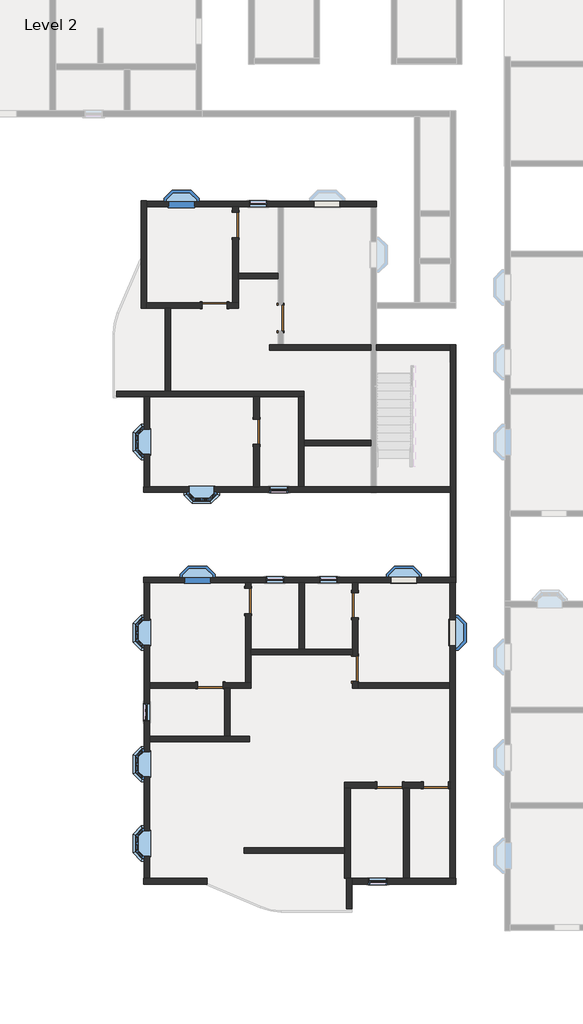
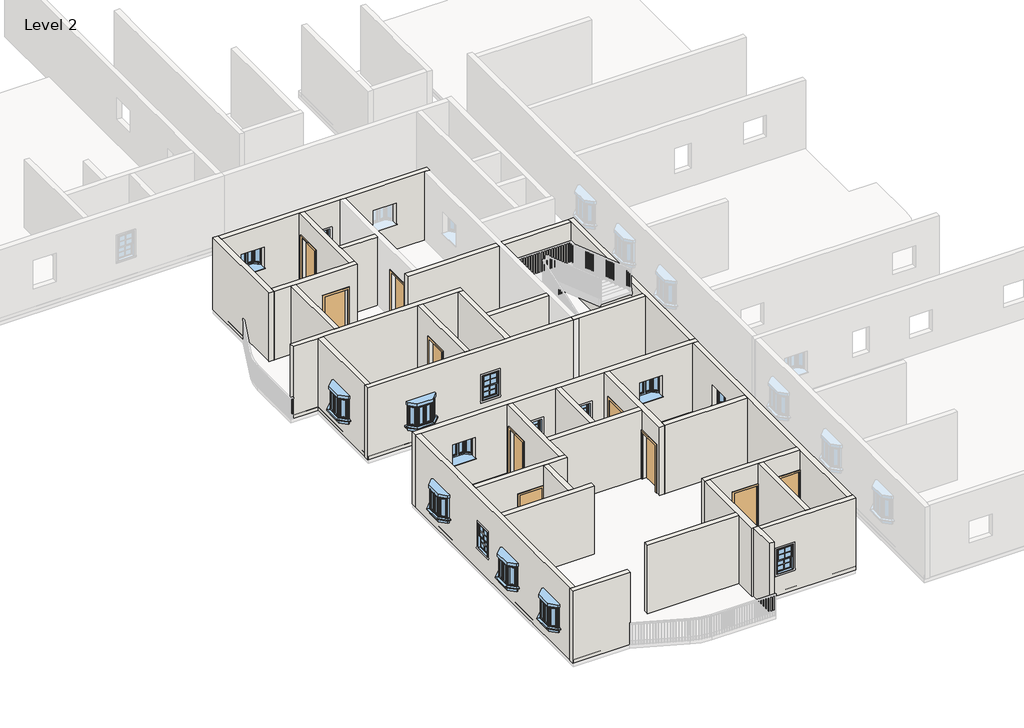
# One storey, part 1 of 14: 32 walls, 15 windows, 10 doors.
"""IFC4 building model written with IfcOpenShell, lengths in millimetres."""

from ifc_helpers import new_model, si_unit, frame, origin, place, context, project, spatial, polyline, outline, extrude, faceted_brep, transform, mapped, element, save
from components import door_54dd4da4, door_719f80de, window_910x910mm_67ef725a, window_8debb0fa

model = new_model("IFC4")

# Units and contexts
model_context = context("Model", 3, world=origin())
ifc_project = project(units=[si_unit("LENGTHUNIT", "METRE", prefix="MILLI")], contexts=[model_context])

# Site, building, storey
site = spatial("IfcSite", under=ifc_project)
building = spatial("IfcBuilding", under=site)
storey = spatial("IfcBuildingStorey", under=building, Name="Level 2", Elevation=3048.0)

# Doors
placement = place(None, origin())
door_shape = door_54dd4da4(model_context)
element("IfcDoor", 1, ObjectType="Single-Flush : 36\" x 84\"", at=placement, inside=storey, context=model_context, shape_type="MappedRepresentation", body=[
    mapped(door_shape, transform((-4626.037215, -17283.4916506, 3048.0), x_axis=(0.0, -1.0, 0.0), y_axis=(1.0, 0.0, 0.0), z_axis=(0.0, 0.0, 1.0))),
])
element("IfcDoor", 2, ObjectType="Single-Flush : 36\" x 84\"", at=placement, inside=storey, context=model_context, shape_type="MappedRepresentation", body=[
    mapped(door_shape, transform((-4626.037215, -14978.4416506, 3048.0), x_axis=(0.0, 1.0, 0.0), y_axis=(-1.0, 0.0, 0.0), z_axis=(0.0, 0.0, 1.0))),
])
element("IfcDoor", 3, ObjectType="Single-Flush : 36\" x 84\"", at=placement, inside=storey, context=model_context, shape_type="MappedRepresentation", body=[
    mapped(door_shape, transform((-9731.437215, -4100.8916506, 3048.0), x_axis=(1.0, 0.0, 0.0), y_axis=(0.0, 1.0, 0.0), z_axis=(0.0, 0.0, 1.0))),
])
element("IfcDoor", 4, ObjectType="Single-Flush : 36\" x 84\"", at=placement, inside=storey, context=model_context, shape_type="MappedRepresentation", body=[
    mapped(door_shape, transform((-7331.137215, -4558.0916506, 3048.0), x_axis=(0.0, -1.0, 0.0), y_axis=(1.0, 0.0, 0.0), z_axis=(0.0, 0.0, 1.0))),
])
door_2_shape = door_719f80de(model_context)
element("IfcDoor", 5, ObjectType="Single-Flush : 36\" x 84\"", at=placement, inside=storey, context=model_context, shape_type="MappedRepresentation", body=[
    mapped(door_2_shape, transform((-9883.837215, -17891.2072331, 3048.0), x_axis=(1.0, 0.0, 0.0), y_axis=(0.0, 1.0, 0.0), z_axis=(0.0, 0.0, 1.0))),
])
element("IfcDoor", 6, ObjectType="Single-Flush : 36\" x 84\"", at=placement, inside=storey, context=model_context, shape_type="MappedRepresentation", body=[
    mapped(door_2_shape, transform((-8512.237215, -14826.0416506, 3048.0), x_axis=(0.0, 1.0, 0.0), y_axis=(-1.0, 0.0, 0.0), z_axis=(0.0, 0.0, 1.0))),
])
element("IfcDoor", 7, ObjectType="Single-Flush : 36\" x 84\"", at=placement, inside=storey, context=model_context, shape_type="MappedRepresentation", body=[
    mapped(door_2_shape, transform((-8207.437215, -8691.9416506, 3048.0), x_axis=(0.0, 1.0, 0.0), y_axis=(-1.0, 0.0, 0.0), z_axis=(0.0, 0.0, 1.0))),
])
element("IfcDoor", 8, ObjectType="Single-Flush : 36\" x 84\"", at=placement, inside=storey, context=model_context, shape_type="MappedRepresentation", body=[
    mapped(door_2_shape, transform((-8969.437215, -1186.2416506, 3048.0), x_axis=(0.0, 1.0, 0.0), y_axis=(-1.0, 0.0, 0.0), z_axis=(0.0, 0.0, 1.0))),
])
element("IfcDoor", 9, ObjectType="Single-Flush : 36\" x 84\"", at=placement, inside=storey, context=model_context, shape_type="MappedRepresentation", body=[
    mapped(door_2_shape, transform((-3374.4891351, -21512.5916506, 3048.0), x_axis=(1.0, 0.0, 0.0), y_axis=(0.0, 1.0, 0.0), z_axis=(0.0, 0.0, 1.0))),
])
element("IfcDoor", 10, ObjectType="Single-Flush : 36\" x 84\"", at=placement, inside=storey, context=model_context, shape_type="MappedRepresentation", body=[
    mapped(door_2_shape, transform((-1698.0891351, -21512.5916506, 3048.0), x_axis=(1.0, 0.0, 0.0), y_axis=(0.0, 1.0, 0.0), z_axis=(0.0, 0.0, 1.0))),
])

# Walls
element("IfcWall", 11, ObjectType="4.5\" p", at=placement, inside=storey, context=model_context, shape_type="Brep", body=[
    faceted_brep([(-9426.637215, -17992.8072331, 5181.6), (-9426.637215, -17992.8072331, 3048.0), (-9375.837215, -17992.8072331, 3048.0), (-9172.637215, -17992.8072331, 3048.0), (-8410.637215, -17992.8072331, 3048.0), (-8410.637215, -17992.8072331, 6096.0), (-9172.637215, -17992.8072331, 6096.0), (-9375.837215, -17992.8072331, 6096.0), (-12087.287215, -17992.8072331, 6096.0), (-12087.287215, -17992.8072331, 3048.0), (-10341.037215, -17992.8072331, 3048.0), (-10341.037215, -17992.8072331, 5181.6), (-8410.637215, -17789.6072331, 3048.0), (-8613.837215, -17789.6072331, 3048.0), (-9426.637215, -17789.6072331, 3048.0), (-9426.637215, -17789.6072331, 5181.6), (-10341.037215, -17789.6072331, 5181.6), (-10341.037215, -17789.6072331, 3048.0), (-12087.287215, -17789.6072331, 3048.0), (-12087.287215, -17789.6072331, 6096.0), (-8613.837215, -17789.6072331, 6096.0), (-8410.637215, -17789.6072331, 6096.0)], [[[0, 1, 2, 3, 4, 5, 6, 7, 8, 9, 10, 11]], [[12, 13, 14, 15, 16, 17, 18, 19, 20, 21]], [[10, 9, 18, 17]], [[4, 3, 2, 1, 14, 13, 12]], [[8, 7, 6, 5, 21, 20, 19]], [[9, 8, 19, 18]], [[5, 4, 12, 21]], [[15, 14, 1, 0]], [[16, 15, 0, 11]], [[17, 16, 11, 10]]]),
])
element("IfcWall", 12, ObjectType="4.5\" p", at=placement, inside=storey, context=model_context, shape_type="Brep", body=[
    faceted_brep([(-8410.637215, -14368.8416506, 5181.6), (-8410.637215, -14368.8416506, 3048.0), (-8410.637215, -14165.6416506, 3048.0), (-8410.637215, -14165.6416506, 6096.0), (-8410.637215, -16572.2916506, 6096.0), (-8410.637215, -16775.4916506, 6096.0), (-8410.637215, -17789.6072331, 6096.0), (-8410.637215, -17789.6072331, 3048.0), (-8410.637215, -16775.4916506, 3048.0), (-8410.637215, -16572.2916506, 3048.0), (-8410.637215, -15283.2416506, 3048.0), (-8410.637215, -15283.2416506, 5181.6), (-8613.837215, -14165.6416506, 3048.0), (-8613.837215, -14368.8416506, 3048.0), (-8613.837215, -14368.8416506, 5181.6), (-8613.837215, -15283.2416506, 5181.6), (-8613.837215, -15283.2416506, 3048.0), (-8613.837215, -17789.6072331, 3048.0), (-8613.837215, -17789.6072331, 6096.0), (-8613.837215, -14165.6416506, 6096.0)], [[[0, 1, 2, 3, 4, 5, 6, 7, 8, 9, 10, 11]], [[12, 13, 14, 15, 16, 17, 18, 19]], [[2, 1, 13, 12]], [[10, 9, 8, 7, 17, 16]], [[6, 5, 4, 3, 19, 18]], [[7, 6, 18, 17]], [[3, 2, 12, 19]], [[14, 13, 1, 0]], [[15, 14, 0, 11]], [[16, 15, 11, 10]]]),
])
element("IfcWall", 13, ObjectType="4.5\" p", at=placement, inside=storey, context=model_context, shape_type="Brep", body=[
    faceted_brep([(-8410.637215, -16775.4916506, 3048.0), (-4727.637215, -16775.4916506, 3048.0), (-4727.637215, -16775.4916506, 6096.0), (-8410.637215, -16775.4916506, 6096.0), (-8410.637215, -16572.2916506, 3048.0), (-8410.637215, -16572.2916506, 6096.0), (-6670.737215, -16572.2916506, 6096.0), (-6467.537215, -16572.2916506, 6096.0), (-4727.637215, -16572.2916506, 6096.0), (-4727.637215, -16572.2916506, 3048.0), (-6467.537215, -16572.2916506, 3048.0), (-6670.737215, -16572.2916506, 3048.0)], [[[0, 1, 2, 3]], [[4, 5, 6, 7, 8, 9, 10, 11]], [[1, 0, 4, 11, 10, 9]], [[3, 2, 8, 7, 6, 5]], [[0, 3, 5, 4]], [[2, 1, 9, 8]]]),
])
element("IfcWall", 14, ObjectType="4.5\" p", at=placement, inside=storey, context=model_context, shape_type="SweptSolid", body=[
    extrude(outline(polyline([(-6670.737215, -16572.2916506), (-6670.737215, -14165.6416506), (-6467.537215, -14165.6416506), (-6467.537215, -16572.2916506), (-6670.737215, -16572.2916506)])), frame((0.0, 0.0, 3048.0), z_axis=(0.0, 0.0, 1.0), x_axis=(1.0, 0.0, 0.0)), (0.0, 0.0, 1.0), 3048.0),
])
element("IfcWall", 15, ObjectType="4.5\" p", at=placement, inside=storey, context=model_context, shape_type="Brep", body=[
    faceted_brep([(-4727.637215, -14165.6416506, 3048.0), (-4727.637215, -14521.2416506, 3048.0), (-4727.637215, -14521.2416506, 5181.6), (-4727.637215, -15435.6416506, 5181.6), (-4727.637215, -15435.6416506, 3048.0), (-4727.637215, -16572.2916506, 3048.0), (-4727.637215, -16775.4916506, 3048.0), (-4727.637215, -16826.2916506, 3048.0), (-4727.637215, -16826.2916506, 5181.6), (-4727.637215, -17740.6916506, 5181.6), (-4727.637215, -17740.6916506, 3048.0), (-4727.637215, -17994.6916506, 3048.0), (-4727.637215, -17994.6916506, 6096.0), (-4727.637215, -16775.4916506, 6096.0), (-4727.637215, -16572.2916506, 6096.0), (-4727.637215, -14165.6416506, 6096.0), (-4524.437215, -14521.2416506, 5181.6), (-4524.437215, -14521.2416506, 3048.0), (-4524.437215, -14165.6416506, 3048.0), (-4524.437215, -14165.6416506, 6096.0), (-4524.437215, -17791.4916506, 6096.0), (-4524.437215, -17994.6916506, 6096.0), (-4524.437215, -17994.6916506, 3048.0), (-4524.437215, -17791.4916506, 3048.0), (-4524.437215, -17740.6916506, 3048.0), (-4524.437215, -17740.6916506, 5181.6), (-4524.437215, -16826.2916506, 5181.6), (-4524.437215, -16826.2916506, 3048.0), (-4524.437215, -15435.6416506, 3048.0), (-4524.437215, -15435.6416506, 5181.6)], [[[0, 1, 2, 3, 4, 5, 6, 7, 8, 9, 10, 11, 12, 13, 14, 15]], [[16, 17, 18, 19, 20, 21, 22, 23, 24, 25, 26, 27, 28, 29]], [[11, 10, 24, 23, 22]], [[28, 27, 7, 6, 5, 4]], [[18, 17, 1, 0]], [[15, 14, 13, 12, 21, 20, 19]], [[0, 15, 19, 18]], [[12, 11, 22, 21]], [[25, 24, 10, 9]], [[26, 25, 9, 8]], [[27, 26, 8, 7]], [[2, 1, 17, 16]], [[3, 2, 16, 29]], [[4, 3, 29, 28]]]),
])
element("IfcWall", 16, ObjectType="4.5\" p", at=placement, inside=storey, context=model_context, shape_type="SweptSolid", body=[
    extrude(outline(polyline([(-4524.437215, -17791.4916506), (-1190.0891351, -17791.4916506), (-1190.0891351, -17994.6916506), (-4524.437215, -17994.6916506), (-4524.437215, -17791.4916506)])), frame((0.0, 0.0, 3048.0), z_axis=(0.0, 0.0, 1.0), x_axis=(1.0, 0.0, 0.0)), (0.0, 0.0, 1.0), 3048.0),
])
element("IfcWall", 17, ObjectType="4.5\" p", at=placement, inside=storey, context=model_context, shape_type="SweptSolid", body=[
    extrude(outline(polyline([(-9375.837215, -19734.5916506), (-9375.837215, -17992.8072331), (-9172.637215, -17992.8072331), (-9172.637215, -19734.5916506), (-9375.837215, -19734.5916506)])), frame((0.0, 0.0, 3048.0), z_axis=(0.0, 0.0, 1.0), x_axis=(1.0, 0.0, 0.0)), (0.0, 0.0, 1.0), 3048.0),
])
element("IfcWall", 18, ObjectType="4.5\" p", at=placement, inside=storey, context=model_context, shape_type="Brep", body=[
    faceted_brep([(-12087.287215, -19937.7916506, 3048.0), (-8455.087215, -19937.7916506, 3048.0), (-8455.087215, -19937.7916506, 6096.0), (-12087.287215, -19937.7916506, 6096.0), (-12087.287215, -19734.5916506, 3048.0), (-12087.287215, -19734.5916506, 6096.0), (-9375.837215, -19734.5916506, 6096.0), (-9172.637215, -19734.5916506, 6096.0), (-8455.087215, -19734.5916506, 6096.0), (-8455.087215, -19734.5916506, 3048.0), (-9172.637215, -19734.5916506, 3048.0), (-9375.837215, -19734.5916506, 3048.0)], [[[0, 1, 2, 3]], [[4, 5, 6, 7, 8, 9, 10, 11]], [[1, 0, 4, 11, 10, 9]], [[2, 1, 9, 8]], [[3, 2, 8, 7, 6, 5]], [[0, 3, 5, 4]]]),
])
element("IfcWall", 19, ObjectType="4.5\" p", at=placement, inside=storey, context=model_context, shape_type="Brep", body=[
    faceted_brep([(-13293.787215, -7421.9416506, 3048.0), (-12290.487215, -7421.9416506, 3048.0), (-12087.287215, -7421.9416506, 3048.0), (-8309.037215, -7421.9416506, 3048.0), (-8105.837215, -7421.9416506, 3048.0), (-6689.787215, -7421.9416506, 3048.0), (-6486.587215, -7421.9416506, 3048.0), (-6486.587215, -7421.9416506, 6096.0), (-6689.787215, -7421.9416506, 6096.0), (-8105.837215, -7421.9416506, 6096.0), (-8309.037215, -7421.9416506, 6096.0), (-12087.287215, -7421.9416506, 6096.0), (-12290.487215, -7421.9416506, 6096.0), (-13293.787215, -7421.9416506, 6096.0), (-13293.787215, -7218.7416506, 3048.0), (-13293.787215, -7218.7416506, 6096.0), (-11528.487215, -7218.7416506, 6096.0), (-11325.287215, -7218.7416506, 6096.0), (-6486.587215, -7218.7416506, 6096.0), (-6486.587215, -7218.7416506, 3048.0), (-11325.287215, -7218.7416506, 3048.0), (-11528.487215, -7218.7416506, 3048.0)], [[[0, 1, 2, 3, 4, 5, 6, 7, 8, 9, 10, 11, 12, 13]], [[14, 15, 16, 17, 18, 19, 20, 21]], [[6, 5, 4, 3, 2, 1, 0, 14, 21, 20, 19]], [[13, 12, 11, 10, 9, 8, 7, 18, 17, 16, 15]], [[0, 13, 15, 14]], [[7, 6, 19, 18]]]),
])
element("IfcWall", 20, ObjectType="4.5\" p", at=placement, inside=storey, context=model_context, shape_type="Brep", body=[
    faceted_brep([(-12201.587215, -4202.4916506, 3048.0), (-12201.587215, -3999.2916506, 3048.0), (-12201.587215, -525.8416506, 3048.0), (-12201.587215, -322.6416506, 3048.0), (-12201.587215, -309.9416506, 3048.0), (-12201.587215, -309.9416506, 6096.0), (-12201.587215, -322.6416506, 6096.0), (-12201.587215, -525.8416506, 6096.0), (-12201.587215, -3999.2916506, 6096.0), (-12201.587215, -4202.4916506, 6096.0), (-12404.787215, -4202.4916506, 3048.0), (-12404.787215, -4202.4916506, 6096.0), (-12404.787215, -309.9416506, 6096.0), (-12404.787215, -309.9416506, 3048.0)], [[[0, 1, 2, 3, 4, 5, 6, 7, 8, 9]], [[10, 11, 12, 13]], [[4, 3, 2, 1, 0, 10, 13]], [[5, 4, 13, 12]], [[9, 8, 7, 6, 5, 12, 11]], [[0, 9, 11, 10]]]),
])
element("IfcWall", 21, ObjectType="4.5\" p", at=placement, inside=storey, context=model_context, shape_type="Brep", body=[
    faceted_brep([(-9274.237215, -4202.4916506, 5181.6), (-9274.237215, -4202.4916506, 3048.0), (-8867.837215, -4202.4916506, 3048.0), (-8867.837215, -4202.4916506, 6096.0), (-11325.287215, -4202.4916506, 6096.0), (-11528.487215, -4202.4916506, 6096.0), (-12201.587215, -4202.4916506, 6096.0), (-12201.587215, -4202.4916506, 3048.0), (-11528.487215, -4202.4916506, 3048.0), (-11325.287215, -4202.4916506, 3048.0), (-10188.637215, -4202.4916506, 3048.0), (-10188.637215, -4202.4916506, 5181.6), (-8867.837215, -3999.2916506, 3048.0), (-9071.037215, -3999.2916506, 3048.0), (-9274.237215, -3999.2916506, 3048.0), (-9274.237215, -3999.2916506, 5181.6), (-10188.637215, -3999.2916506, 5181.6), (-10188.637215, -3999.2916506, 3048.0), (-12201.587215, -3999.2916506, 3048.0), (-12201.587215, -3999.2916506, 6096.0), (-9071.037215, -3999.2916506, 6096.0), (-8867.837215, -3999.2916506, 6096.0)], [[[0, 1, 2, 3, 4, 5, 6, 7, 8, 9, 10, 11]], [[12, 13, 14, 15, 16, 17, 18, 19, 20, 21]], [[2, 1, 14, 13, 12]], [[10, 9, 8, 7, 18, 17]], [[6, 5, 4, 3, 21, 20, 19]], [[7, 6, 19, 18]], [[3, 2, 12, 21]], [[15, 14, 1, 0]], [[16, 15, 0, 11]], [[17, 16, 11, 10]]]),
])
element("IfcWall", 22, ObjectType="4.5\" p", at=placement, inside=storey, context=model_context, shape_type="Brep", body=[
    faceted_brep([(-8867.837215, -729.0416506, 5181.6), (-8867.837215, -729.0416506, 3048.0), (-8867.837215, -525.8416506, 3048.0), (-8867.837215, -525.8416506, 6096.0), (-8867.837215, -2932.4916506, 6096.0), (-8867.837215, -3135.6916506, 6096.0), (-8867.837215, -3999.2916506, 6096.0), (-8867.837215, -3999.2916506, 3048.0), (-8867.837215, -3135.6916506, 3048.0), (-8867.837215, -2932.4916506, 3048.0), (-8867.837215, -1643.4416506, 3048.0), (-8867.837215, -1643.4416506, 5181.6), (-9071.037215, -525.8416506, 3048.0), (-9071.037215, -729.0416506, 3048.0), (-9071.037215, -729.0416506, 5181.6), (-9071.037215, -1643.4416506, 5181.6), (-9071.037215, -1643.4416506, 3048.0), (-9071.037215, -3999.2916506, 3048.0), (-9071.037215, -3999.2916506, 6096.0), (-9071.037215, -525.8416506, 6096.0)], [[[0, 1, 2, 3, 4, 5, 6, 7, 8, 9, 10, 11]], [[12, 13, 14, 15, 16, 17, 18, 19]], [[2, 1, 13, 12]], [[10, 9, 8, 7, 17, 16]], [[6, 5, 4, 3, 19, 18]], [[7, 6, 18, 17]], [[3, 2, 12, 19]], [[14, 13, 1, 0]], [[15, 14, 0, 11]], [[16, 15, 11, 10]]]),
])
element("IfcWall", 23, ObjectType="4.5\" p", at=placement, inside=storey, context=model_context, shape_type="SweptSolid", body=[
    extrude(outline(polyline([(-7432.737215, -3135.6916506), (-8867.837215, -3135.6916506), (-8867.837215, -2932.4916506), (-7432.737215, -2932.4916506), (-7432.737215, -3135.6916506)])), frame((0.0, 0.0, 3048.0), z_axis=(0.0, 0.0, 1.0), x_axis=(1.0, 0.0, 0.0)), (0.0, 0.0, 1.0), 3048.0),
])
element("IfcWall", 24, ObjectType="4.5\" p", at=placement, inside=storey, context=model_context, shape_type="Brep", body=[
    faceted_brep([(-7731.187215, -5726.4916506, 6096.0), (-7731.187215, -5726.4916506, 3048.0), (-4060.887215, -5726.4916506, 3048.0), (-4060.887215, -5726.4916506, 6096.0), (-7731.187215, -5523.2916506, 3048.0), (-7731.187215, -5523.2916506, 6096.0), (-7432.737215, -5523.2916506, 6096.0), (-7229.537215, -5523.2916506, 6096.0), (-4060.887215, -5523.2916506, 6096.0), (-4060.887215, -5523.2916506, 3048.0), (-7229.537215, -5523.2916506, 3048.0), (-7432.737215, -5523.2916506, 3048.0)], [[[0, 1, 2, 3]], [[4, 5, 6, 7, 8, 9, 10, 11]], [[1, 4, 11, 10, 9, 2]], [[5, 0, 3, 8, 7, 6]], [[1, 0, 5, 4]], [[3, 2, 9, 8]]]),
    faceted_brep([(-1177.3891351, -5726.4916506, 3048.0), (-1177.3891351, -5726.4916506, 6096.0), (-3857.687215, -5726.4916506, 6096.0), (-3857.687215, -5726.4916506, 3048.0), (-1177.3891351, -5523.2916506, 6096.0), (-1177.3891351, -5523.2916506, 3048.0), (-3857.687215, -5523.2916506, 3048.0), (-3857.687215, -5523.2916506, 6096.0)], [[[0, 1, 2, 3]], [[4, 5, 6, 7]], [[5, 0, 3, 6]], [[1, 4, 7, 2]], [[1, 0, 5, 4]], [[3, 2, 7, 6]]]),
])
element("IfcWall", 25, ObjectType="4.5\" p", at=placement, inside=storey, context=model_context, shape_type="SweptSolid", body=[
    extrude(outline(polyline([(-11528.487215, -7218.7416506), (-11528.487215, -4202.4916506), (-11325.287215, -4202.4916506), (-11325.287215, -7218.7416506), (-11528.487215, -7218.7416506)])), frame((0.0, 0.0, 3048.0), z_axis=(0.0, 0.0, 1.0), x_axis=(1.0, 0.0, 0.0)), (0.0, 0.0, 1.0), 3048.0),
])
element("IfcWall", 26, ObjectType="4.5\" p", at=placement, inside=storey, context=model_context, shape_type="SweptSolid", body=[
    extrude(outline(polyline([(-7421.9416506, 3048.0), (-8234.7416506, 3048.0), (-8234.7416506, 5181.6), (-9149.1416506, 5181.6), (-9149.1416506, 3048.0), (-10685.8416506, 3048.0), (-10685.8416506, 6096.0), (-7421.9416506, 6096.0), (-7421.9416506, 3048.0)])), frame((-8309.037215, 0.0, 0.0), z_axis=(1.0, 0.0, 0.0), x_axis=(0.0, 1.0, 0.0)), (0.0, 0.0, 1.0), 203.2),
])
element("IfcWall", 27, ObjectType="4.5\" p", at=placement, inside=storey, context=model_context, shape_type="Brep", body=[
    faceted_brep([(-6689.787215, -7421.9416506, 3048.0), (-6689.787215, -10685.8416506, 3048.0), (-6689.787215, -10685.8416506, 6096.0), (-6689.787215, -7421.9416506, 6096.0), (-6486.587215, -7421.9416506, 3048.0), (-6486.587215, -7421.9416506, 6096.0), (-6486.587215, -8990.3916506, 6096.0), (-6486.587215, -9193.5916506, 6096.0), (-6486.587215, -10685.8416506, 6096.0), (-6486.587215, -10685.8416506, 3048.0), (-6486.587215, -9193.5916506, 3048.0), (-6486.587215, -8990.3916506, 3048.0)], [[[0, 1, 2, 3]], [[4, 5, 6, 7, 8, 9, 10, 11]], [[1, 0, 4, 11, 10, 9]], [[3, 2, 8, 7, 6, 5]], [[0, 3, 5, 4]], [[2, 1, 9, 8]]]),
])
element("IfcWall", 28, ObjectType="4.5\" p", at=placement, inside=storey, context=model_context, shape_type="SweptSolid", body=[
    extrude(outline(polyline([(-4060.887215, -9193.5916506), (-6486.587215, -9193.5916506), (-6486.587215, -8990.3916506), (-4060.887215, -8990.3916506), (-4060.887215, -9193.5916506)])), frame((0.0, 0.0, 3048.0), z_axis=(0.0, 0.0, 1.0), x_axis=(1.0, 0.0, 0.0)), (0.0, 0.0, 1.0), 3048.0),
])
element("IfcWall", 29, ObjectType="9\"", at=placement, inside=storey, context=model_context, shape_type="Brep", body=[
    faceted_brep([(-1190.0891351, -21410.9916506, 3048.0), (-1240.8891351, -21410.9916506, 3048.0), (-1240.8891351, -21410.9916506, 5181.6), (-2155.2891351, -21410.9916506, 5181.6), (-2155.2891351, -21410.9916506, 3048.0), (-2917.2891351, -21410.9916506, 3048.0), (-2917.2891351, -21410.9916506, 5181.6), (-3831.6891351, -21410.9916506, 5181.6), (-3831.6891351, -21410.9916506, 3048.0), (-5006.4391351, -21410.9916506, 3048.0), (-5006.4391351, -21410.9916506, 6096.0), (-1190.0891351, -21410.9916506, 6096.0), (-1240.8891351, -21614.1916506, 5181.6), (-1240.8891351, -21614.1916506, 3048.0), (-1190.0891351, -21614.1916506, 3048.0), (-1190.0891351, -21614.1916506, 6096.0), (-2663.2891351, -21614.1916506, 6096.0), (-2866.4891351, -21614.1916506, 6096.0), (-4803.2391351, -21614.1916506, 6096.0), (-5006.4391351, -21614.1916506, 6096.0), (-5006.4391351, -21614.1916506, 3048.0), (-4803.2391351, -21614.1916506, 3048.0), (-3831.6891351, -21614.1916506, 3048.0), (-3831.6891351, -21614.1916506, 5181.6), (-2917.2891351, -21614.1916506, 5181.6), (-2917.2891351, -21614.1916506, 3048.0), (-2866.4891351, -21614.1916506, 3048.0), (-2663.2891351, -21614.1916506, 3048.0), (-2155.2891351, -21614.1916506, 3048.0), (-2155.2891351, -21614.1916506, 5181.6)], [[[0, 1, 2, 3, 4, 5, 6, 7, 8, 9, 10, 11]], [[12, 13, 14, 15, 16, 17, 18, 19, 20, 21, 22, 23, 24, 25, 26, 27, 28, 29]], [[22, 21, 20, 9, 8]], [[14, 13, 1, 0]], [[28, 27, 26, 25, 5, 4]], [[11, 10, 19, 18, 17, 16, 15]], [[0, 11, 15, 14]], [[10, 9, 20, 19]], [[6, 5, 25, 24]], [[7, 6, 24, 23]], [[8, 7, 23, 22]], [[2, 1, 13, 12]], [[3, 2, 12, 29]], [[4, 3, 29, 28]]]),
])
element("IfcWall", 30, ObjectType="9\"", at=placement, inside=storey, context=model_context, shape_type="Brep", body=[
    faceted_brep([(-5006.4391351, -21614.1916506, 3048.0), (-5006.4391351, -23779.5416506, 3048.0), (-5006.4391351, -23982.7416506, 3048.0), (-5006.4391351, -24897.1416506, 3048.0), (-5006.4391351, -24897.1416506, 6096.0), (-5006.4391351, -23982.7416506, 6096.0), (-5006.4391351, -23779.5416506, 6096.0), (-5006.4391351, -21614.1916506, 6096.0), (-4803.2391351, -21614.1916506, 3048.0), (-4803.2391351, -21614.1916506, 6096.0), (-4803.2391351, -24897.1416506, 6096.0), (-4803.2391351, -24897.1416506, 3048.0), (-4949.2891351, -24897.1416506, 3048.0), (-4949.2891351, -24897.1416506, 6096.0)], [[[0, 1, 2, 3, 4, 5, 6, 7]], [[8, 9, 10, 11]], [[3, 2, 1, 0, 8, 11, 12]], [[7, 6, 5, 4, 13, 10, 9]], [[0, 7, 9, 8]], [[4, 3, 12, 11, 10, 13]]]),
])
element("IfcWall", 31, ObjectType="9\"", at=placement, inside=storey, context=model_context, shape_type="SweptSolid", body=[
    extrude(outline(polyline([(-2866.4891351, -24897.1416506), (-2866.4891351, -21614.1916506), (-2663.2891351, -21614.1916506), (-2663.2891351, -24897.1416506), (-2866.4891351, -24897.1416506)])), frame((0.0, 0.0, 3048.0), z_axis=(0.0, 0.0, 1.0), x_axis=(1.0, 0.0, 0.0)), (0.0, 0.0, 1.0), 3048.0),
])
element("IfcWall", 32, ObjectType="9\"", at=placement, inside=storey, context=model_context, shape_type="SweptSolid", body=[
    extrude(outline(polyline([(-5006.4391351, -23982.7416506), (-8664.637215, -23982.7416506), (-8664.637215, -23779.5416506), (-5006.4391351, -23779.5416506), (-5006.4391351, -23982.7416506)])), frame((0.0, 0.0, 3048.0), z_axis=(0.0, 0.0, 1.0), x_axis=(1.0, 0.0, 0.0)), (0.0, 0.0, 1.0), 3048.0),
])
element("IfcWall", 33, ObjectType="9\" w", at=placement, inside=storey, context=model_context, shape_type="Brep", body=[
    faceted_brep([(-12303.187215, -14165.6416506, 3048.0), (-12290.487215, -14165.6416506, 3048.0), (-12087.287215, -14165.6416506, 3048.0), (-8613.837215, -14165.6416506, 3048.0), (-8410.637215, -14165.6416506, 3048.0), (-6670.737215, -14165.6416506, 3048.0), (-6467.537215, -14165.6416506, 3048.0), (-4727.637215, -14165.6416506, 3048.0), (-4524.437215, -14165.6416506, 3048.0), (-1190.0891351, -14165.6416506, 3048.0), (-986.8891351, -14165.6416506, 3048.0), (-961.4891351, -14165.6416506, 3048.0), (-961.4891351, -14165.6416506, 6096.0), (-986.8891351, -14165.6416506, 6096.0), (-1190.0891351, -14165.6416506, 6096.0), (-4524.437215, -14165.6416506, 6096.0), (-4727.637215, -14165.6416506, 6096.0), (-6467.537215, -14165.6416506, 6096.0), (-6670.737215, -14165.6416506, 6096.0), (-8410.637215, -14165.6416506, 6096.0), (-8613.837215, -14165.6416506, 6096.0), (-12087.287215, -14165.6416506, 6096.0), (-12290.487215, -14165.6416506, 6096.0), (-12303.187215, -14165.6416506, 6096.0), (-10805.562215, -14165.6416506, 5158.0), (-9895.562215, -14165.6416506, 5158.0), (-9895.562215, -14165.6416506, 4248.0), (-10805.562215, -14165.6416506, 4248.0), (-3312.2631751, -14165.6416506, 5158.0), (-2402.2631751, -14165.6416506, 5158.0), (-2402.2631751, -14165.6416506, 4248.0), (-3312.2631751, -14165.6416506, 4248.0), (-7870.887215, -14165.6416506, 5029.2), (-7210.487215, -14165.6416506, 5029.2), (-7210.487215, -14165.6416506, 3962.4), (-7870.887215, -14165.6416506, 3962.4), (-5927.787215, -14165.6416506, 5029.2), (-5267.387215, -14165.6416506, 5029.2), (-5267.387215, -14165.6416506, 3962.4), (-5927.787215, -14165.6416506, 3962.4), (-12303.187215, -13962.4416506, 3048.0), (-12303.187215, -13962.4416506, 6096.0), (-1177.3891351, -13962.4416506, 6096.0), (-974.1891351, -13962.4416506, 6096.0), (-961.4891351, -13962.4416506, 6096.0), (-961.4891351, -13962.4416506, 3048.0), (-974.1891351, -13962.4416506, 3048.0), (-1177.3891351, -13962.4416506, 3048.0), (-10805.562215, -13962.4416506, 5158.0), (-10805.562215, -13962.4416506, 4248.0), (-9895.562215, -13962.4416506, 4248.0), (-9895.562215, -13962.4416506, 5158.0), (-3312.2631751, -13962.4416506, 5158.0), (-3312.2631751, -13962.4416506, 4248.0), (-2402.2631751, -13962.4416506, 4248.0), (-2402.2631751, -13962.4416506, 5158.0), (-7870.887215, -13962.4416506, 5029.2), (-7870.887215, -13962.4416506, 3962.4), (-7210.487215, -13962.4416506, 3962.4), (-7210.487215, -13962.4416506, 5029.2), (-5927.787215, -13962.4416506, 5029.2), (-5927.787215, -13962.4416506, 3962.4), (-5267.387215, -13962.4416506, 3962.4), (-5267.387215, -13962.4416506, 5029.2)], [[[0, 1, 2, 3, 4, 5, 6, 7, 8, 9, 10, 11, 12, 13, 14, 15, 16, 17, 18, 19, 20, 21, 22, 23], [24, 25, 26, 27], [28, 29, 30, 31], [32, 33, 34, 35], [36, 37, 38, 39]], [[40, 41, 42, 43, 44, 45, 46, 47], [48, 49, 50, 51], [52, 53, 54, 55], [56, 57, 58, 59], [60, 61, 62, 63]], [[11, 10, 9, 8, 7, 6, 5, 4, 3, 2, 1, 0, 40, 47, 46, 45]], [[12, 11, 45, 44]], [[23, 22, 21, 20, 19, 18, 17, 16, 15, 14, 13, 12, 44, 43, 42, 41]], [[0, 23, 41, 40]], [[49, 48, 24, 27]], [[50, 49, 27, 26]], [[51, 50, 26, 25]], [[48, 51, 25, 24]], [[53, 52, 28, 31]], [[54, 53, 31, 30]], [[55, 54, 30, 29]], [[52, 55, 29, 28]], [[57, 56, 32, 35]], [[58, 57, 35, 34]], [[59, 58, 34, 33]], [[56, 59, 33, 32]], [[61, 60, 36, 39]], [[62, 61, 39, 38]], [[63, 62, 38, 37]], [[60, 63, 37, 36]]]),
])
element("IfcWall", 34, ObjectType="9\" w", at=placement, inside=storey, context=model_context, shape_type="Brep", body=[
    faceted_brep([(-10004.0323936, -24897.1416506, 3048.0), (-12087.287215, -24897.1416506, 3048.0), (-12290.487215, -24897.1416506, 3048.0), (-12303.187215, -24897.1416506, 3048.0), (-12303.187215, -24897.1416506, 6096.0), (-12290.487215, -24897.1416506, 6096.0), (-12087.287215, -24897.1416506, 6096.0), (-10004.0323936, -24897.1416506, 6096.0), (-10004.0323936, -25100.3416506, 3048.0), (-10004.0323936, -25100.3416506, 6096.0), (-12303.187215, -25100.3416506, 6096.0), (-12303.187215, -25100.3416506, 3048.0)], [[[0, 1, 2, 3, 4, 5, 6, 7]], [[8, 9, 10, 11]], [[3, 2, 1, 0, 8, 11]], [[4, 3, 11, 10]], [[7, 6, 5, 4, 10, 9]], [[0, 7, 9, 8]]]),
])
element("IfcWall", 35, ObjectType="9\" w", at=placement, inside=storey, context=model_context, shape_type="Brep", body=[
    faceted_brep([(-4746.0891351, -25989.3416506, 3048.0), (-4746.0891351, -25100.3416506, 3048.0), (-4746.0891351, -24897.1416506, 3048.0), (-4746.0891351, -24897.1416506, 6096.0), (-4746.0891351, -25100.3416506, 6096.0), (-4746.0891351, -25989.3416506, 6096.0), (-4949.2891351, -25989.3416506, 3048.0), (-4949.2891351, -25989.3416506, 6096.0), (-4949.2891351, -24897.1416506, 6096.0), (-4949.2891351, -24897.1416506, 3048.0), (-4803.2391351, -24897.1416506, 3048.0), (-4803.2391351, -24897.1416506, 6096.0)], [[[0, 1, 2, 3, 4, 5]], [[6, 7, 8, 9]], [[2, 1, 0, 6, 9, 10]], [[5, 4, 3, 11, 8, 7]], [[0, 5, 7, 6]], [[3, 2, 10, 9, 8, 11]]]),
])
element("IfcWall", 36, ObjectType="9\" w", at=placement, inside=storey, context=model_context, shape_type="Brep", body=[
    faceted_brep([(-4746.0891351, -25100.3416506, 3048.0), (-961.4891351, -25100.3416506, 3048.0), (-961.4891351, -25100.3416506, 6096.0), (-4746.0891351, -25100.3416506, 6096.0), (-3476.0891351, -25100.3416506, 5029.2), (-3476.0891351, -25100.3416506, 3962.4), (-4136.4891351, -25100.3416506, 3962.4), (-4136.4891351, -25100.3416506, 5029.2), (-4746.0891351, -24897.1416506, 3048.0), (-4746.0891351, -24897.1416506, 6096.0), (-2866.4891351, -24897.1416506, 6096.0), (-2663.2891351, -24897.1416506, 6096.0), (-1190.0891351, -24897.1416506, 6096.0), (-986.8891351, -24897.1416506, 6096.0), (-961.4891351, -24897.1416506, 6096.0), (-961.4891351, -24897.1416506, 3048.0), (-986.8891351, -24897.1416506, 3048.0), (-1190.0891351, -24897.1416506, 3048.0), (-2663.2891351, -24897.1416506, 3048.0), (-2866.4891351, -24897.1416506, 3048.0), (-3476.0891351, -24897.1416506, 5029.2), (-4136.4891351, -24897.1416506, 5029.2), (-4136.4891351, -24897.1416506, 3962.4), (-3476.0891351, -24897.1416506, 3962.4)], [[[0, 1, 2, 3], [4, 5, 6, 7]], [[8, 9, 10, 11, 12, 13, 14, 15, 16, 17, 18, 19], [20, 21, 22, 23]], [[1, 0, 8, 19, 18, 17, 16, 15]], [[2, 1, 15, 14]], [[3, 2, 14, 13, 12, 11, 10, 9]], [[0, 3, 9, 8]], [[5, 4, 20, 23]], [[6, 5, 23, 22]], [[7, 6, 22, 21]], [[4, 7, 21, 20]]]),
])
element("IfcWall", 37, ObjectType="9\" w", at=placement, inside=storey, context=model_context, shape_type="Brep", body=[
    faceted_brep([(-12290.487215, -14165.6416506, 3048.0), (-12290.487215, -24897.1416506, 3048.0), (-12290.487215, -24897.1416506, 6096.0), (-12290.487215, -14165.6416506, 6096.0), (-12290.487215, -16432.6244419, 4872.4), (-12290.487215, -16432.6244419, 3962.4), (-12290.487215, -15522.6244419, 3962.4), (-12290.487215, -15522.6244419, 4872.4), (-12290.487215, -21205.5916506, 4872.4), (-12290.487215, -21205.5916506, 3962.4), (-12290.487215, -20295.5916506, 3962.4), (-12290.487215, -20295.5916506, 4872.4), (-12290.487215, -24082.1416506, 4872.4), (-12290.487215, -24082.1416506, 3962.4), (-12290.487215, -23172.1416506, 3962.4), (-12290.487215, -23172.1416506, 4872.4), (-12290.487215, -19193.8994419, 5029.2), (-12290.487215, -19193.8994419, 3962.4), (-12290.487215, -18533.4994419, 3962.4), (-12290.487215, -18533.4994419, 5029.2), (-12087.287215, -14165.6416506, 3048.0), (-12087.287215, -14165.6416506, 6096.0), (-12087.287215, -17789.6072331, 6096.0), (-12087.287215, -17992.8072331, 6096.0), (-12087.287215, -19734.5916506, 6096.0), (-12087.287215, -19937.7916506, 6096.0), (-12087.287215, -24897.1416506, 6096.0), (-12087.287215, -24897.1416506, 3048.0), (-12087.287215, -19937.7916506, 3048.0), (-12087.287215, -19734.5916506, 3048.0), (-12087.287215, -17992.8072331, 3048.0), (-12087.287215, -17789.6072331, 3048.0), (-12087.287215, -16432.6244419, 4872.4), (-12087.287215, -15522.6244419, 4872.4), (-12087.287215, -15522.6244419, 3962.4), (-12087.287215, -16432.6244419, 3962.4), (-12087.287215, -21205.5916506, 4872.4), (-12087.287215, -20295.5916506, 4872.4), (-12087.287215, -20295.5916506, 3962.4), (-12087.287215, -21205.5916506, 3962.4), (-12087.287215, -24082.1416506, 4872.4), (-12087.287215, -23172.1416506, 4872.4), (-12087.287215, -23172.1416506, 3962.4), (-12087.287215, -24082.1416506, 3962.4), (-12087.287215, -19193.8994419, 5029.2), (-12087.287215, -18533.4994419, 5029.2), (-12087.287215, -18533.4994419, 3962.4), (-12087.287215, -19193.8994419, 3962.4)], [[[0, 1, 2, 3], [4, 5, 6, 7], [8, 9, 10, 11], [12, 13, 14, 15], [16, 17, 18, 19]], [[20, 21, 22, 23, 24, 25, 26, 27, 28, 29, 30, 31], [32, 33, 34, 35], [36, 37, 38, 39], [40, 41, 42, 43], [44, 45, 46, 47]], [[1, 0, 20, 31, 30, 29, 28, 27]], [[3, 2, 26, 25, 24, 23, 22, 21]], [[0, 3, 21, 20]], [[2, 1, 27, 26]], [[5, 4, 32, 35]], [[6, 5, 35, 34]], [[7, 6, 34, 33]], [[4, 7, 33, 32]], [[9, 8, 36, 39]], [[10, 9, 39, 38]], [[11, 10, 38, 37]], [[8, 11, 37, 36]], [[13, 12, 40, 43]], [[14, 13, 43, 42]], [[15, 14, 42, 41]], [[12, 15, 41, 40]], [[17, 16, 44, 47]], [[18, 17, 47, 46]], [[19, 18, 46, 45]], [[16, 19, 45, 44]]]),
])
element("IfcWall", 38, ObjectType="9\" w", at=placement, inside=storey, context=model_context, shape_type="Brep", body=[
    faceted_brep([(-1190.0891351, -14165.6416506, 3048.0), (-1190.0891351, -17791.4916506, 3048.0), (-1190.0891351, -17994.6916506, 3048.0), (-1190.0891351, -21410.9916506, 3048.0), (-1190.0891351, -21614.1916506, 3048.0), (-1190.0891351, -24897.1416506, 3048.0), (-1190.0891351, -24897.1416506, 6096.0), (-1190.0891351, -21614.1916506, 6096.0), (-1190.0891351, -21410.9916506, 6096.0), (-1190.0891351, -17994.6916506, 6096.0), (-1190.0891351, -17791.4916506, 6096.0), (-1190.0891351, -14165.6416506, 6096.0), (-1190.0891351, -15523.5666506, 5158.0), (-1190.0891351, -16433.5666506, 5158.0), (-1190.0891351, -16433.5666506, 4248.0), (-1190.0891351, -15523.5666506, 4248.0), (-986.8891351, -14165.6416506, 3048.0), (-986.8891351, -14165.6416506, 6096.0), (-986.8891351, -24897.1416506, 6096.0), (-986.8891351, -24897.1416506, 3048.0), (-986.8891351, -15523.5666506, 5158.0), (-986.8891351, -15523.5666506, 4248.0), (-986.8891351, -16433.5666506, 4248.0), (-986.8891351, -16433.5666506, 5158.0)], [[[0, 1, 2, 3, 4, 5, 6, 7, 8, 9, 10, 11], [12, 13, 14, 15]], [[16, 17, 18, 19], [20, 21, 22, 23]], [[5, 4, 3, 2, 1, 0, 16, 19]], [[11, 10, 9, 8, 7, 6, 18, 17]], [[0, 11, 17, 16]], [[6, 5, 19, 18]], [[21, 20, 12, 15]], [[22, 21, 15, 14]], [[23, 22, 14, 13]], [[20, 23, 13, 12]]]),
])
element("IfcWall", 39, ObjectType="9\" w", at=placement, inside=storey, context=model_context, shape_type="Brep", body=[
    faceted_brep([(-1177.3891351, -5523.2916506, 3048.0), (-1177.3891351, -5726.4916506, 3048.0), (-1177.3891351, -10685.8416506, 3048.0), (-1177.3891351, -10889.0416506, 3048.0), (-1177.3891351, -13962.4416506, 3048.0), (-1177.3891351, -13962.4416506, 6096.0), (-1177.3891351, -10889.0416506, 6096.0), (-1177.3891351, -10685.8416506, 6096.0), (-1177.3891351, -5726.4916506, 6096.0), (-1177.3891351, -5523.2916506, 6096.0), (-974.1891351, -5523.2916506, 3048.0), (-974.1891351, -5523.2916506, 6096.0), (-974.1891351, -13962.4416506, 6096.0), (-974.1891351, -13962.4416506, 3048.0)], [[[0, 1, 2, 3, 4, 5, 6, 7, 8, 9]], [[10, 11, 12, 13]], [[4, 3, 2, 1, 0, 10, 13]], [[9, 8, 7, 6, 5, 12, 11]], [[5, 4, 13, 12]], [[0, 9, 11, 10]]]),
])
element("IfcWall", 40, ObjectType="9\" w", at=placement, inside=storey, context=model_context, shape_type="Brep", body=[
    faceted_brep([(-1177.3891351, -10685.8416506, 3048.0), (-6486.587215, -10685.8416506, 3048.0), (-6689.787215, -10685.8416506, 3048.0), (-8105.837215, -10685.8416506, 3048.0), (-8309.037215, -10685.8416506, 3048.0), (-12087.287215, -10685.8416506, 3048.0), (-12290.487215, -10685.8416506, 3048.0), (-12303.187215, -10685.8416506, 3048.0), (-12303.187215, -10685.8416506, 6096.0), (-12290.487215, -10685.8416506, 6096.0), (-12087.287215, -10685.8416506, 6096.0), (-8309.037215, -10685.8416506, 6096.0), (-8105.837215, -10685.8416506, 6096.0), (-6689.787215, -10685.8416506, 6096.0), (-6486.587215, -10685.8416506, 6096.0), (-1177.3891351, -10685.8416506, 6096.0), (-9743.162215, -10685.8416506, 4872.4), (-10653.162215, -10685.8416506, 4872.4), (-10653.162215, -10685.8416506, 3962.4), (-9743.162215, -10685.8416506, 3962.4), (-7067.612215, -10685.8416506, 5029.2), (-7728.012215, -10685.8416506, 5029.2), (-7728.012215, -10685.8416506, 3962.4), (-7067.612215, -10685.8416506, 3962.4), (-1177.3891351, -10889.0416506, 3048.0), (-1177.3891351, -10889.0416506, 6096.0), (-12303.187215, -10889.0416506, 6096.0), (-12303.187215, -10889.0416506, 3048.0), (-9743.162215, -10889.0416506, 4872.4), (-9743.162215, -10889.0416506, 3962.4), (-10653.162215, -10889.0416506, 3962.4), (-10653.162215, -10889.0416506, 4872.4), (-7067.612215, -10889.0416506, 5029.2), (-7067.612215, -10889.0416506, 3962.4), (-7728.012215, -10889.0416506, 3962.4), (-7728.012215, -10889.0416506, 5029.2)], [[[0, 1, 2, 3, 4, 5, 6, 7, 8, 9, 10, 11, 12, 13, 14, 15], [16, 17, 18, 19], [20, 21, 22, 23]], [[24, 25, 26, 27], [28, 29, 30, 31], [32, 33, 34, 35]], [[7, 6, 5, 4, 3, 2, 1, 0, 24, 27]], [[8, 7, 27, 26]], [[15, 14, 13, 12, 11, 10, 9, 8, 26, 25]], [[0, 15, 25, 24]], [[29, 28, 16, 19]], [[30, 29, 19, 18]], [[31, 30, 18, 17]], [[28, 31, 17, 16]], [[33, 32, 20, 23]], [[34, 33, 23, 22]], [[35, 34, 22, 21]], [[32, 35, 21, 20]]]),
])
element("IfcWall", 41, ObjectType="9\" w", at=placement, inside=storey, context=model_context, shape_type="SweptSolid", body=[
    extrude(outline(polyline([(-10685.8416506, 3048.0), (-10685.8416506, 6096.0), (-7421.9416506, 6096.0), (-7421.9416506, 3048.0), (-10685.8416506, 3048.0)]), holes=[polyline([(-9508.8916506, 4872.4), (-9508.8916506, 3962.4), (-8598.8916506, 3962.4), (-8598.8916506, 4872.4), (-9508.8916506, 4872.4)])]), frame((-12290.487215, 0.0, 0.0), z_axis=(1.0, 0.0, 0.0), x_axis=(0.0, 1.0, 0.0)), (0.0, 0.0, 1.0), 203.2),
])
element("IfcWall", 42, ObjectType="9\" w", at=placement, inside=storey, context=model_context, shape_type="Brep", body=[
    faceted_brep([(-12201.587215, -525.8416506, 3048.0), (-9071.037215, -525.8416506, 3048.0), (-8867.837215, -525.8416506, 3048.0), (-7432.737215, -525.8416506, 3048.0), (-7229.537215, -525.8416506, 3048.0), (-4060.887215, -525.8416506, 3048.0), (-3857.687215, -525.8416506, 3048.0), (-3844.987215, -525.8416506, 3048.0), (-3844.987215, -525.8416506, 6096.0), (-3857.687215, -525.8416506, 6096.0), (-4060.887215, -525.8416506, 6096.0), (-7229.537215, -525.8416506, 6096.0), (-7432.737215, -525.8416506, 6096.0), (-8867.837215, -525.8416506, 6096.0), (-9071.037215, -525.8416506, 6096.0), (-12201.587215, -525.8416506, 6096.0), (-6100.212215, -525.8416506, 5158.0), (-5190.212215, -525.8416506, 5158.0), (-5190.212215, -525.8416506, 4248.0), (-6100.212215, -525.8416506, 4248.0), (-11386.587215, -525.8416506, 5158.0), (-10476.587215, -525.8416506, 5158.0), (-10476.587215, -525.8416506, 4248.0), (-11386.587215, -525.8416506, 4248.0), (-8480.487215, -525.8416506, 5029.2), (-7820.087215, -525.8416506, 5029.2), (-7820.087215, -525.8416506, 3962.4), (-8480.487215, -525.8416506, 3962.4), (-12201.587215, -322.6416506, 3048.0), (-12201.587215, -322.6416506, 6096.0), (-3844.987215, -322.6416506, 6096.0), (-3844.987215, -322.6416506, 3048.0), (-6100.212215, -322.6416506, 5158.0), (-6100.212215, -322.6416506, 4248.0), (-5190.212215, -322.6416506, 4248.0), (-5190.212215, -322.6416506, 5158.0), (-11386.587215, -322.6416506, 5158.0), (-11386.587215, -322.6416506, 4248.0), (-10476.587215, -322.6416506, 4248.0), (-10476.587215, -322.6416506, 5158.0), (-8480.487215, -322.6416506, 5029.2), (-8480.487215, -322.6416506, 3962.4), (-7820.087215, -322.6416506, 3962.4), (-7820.087215, -322.6416506, 5029.2)], [[[0, 1, 2, 3, 4, 5, 6, 7, 8, 9, 10, 11, 12, 13, 14, 15], [16, 17, 18, 19], [20, 21, 22, 23], [24, 25, 26, 27]], [[28, 29, 30, 31], [32, 33, 34, 35], [36, 37, 38, 39], [40, 41, 42, 43]], [[7, 6, 5, 4, 3, 2, 1, 0, 28, 31]], [[8, 7, 31, 30]], [[15, 14, 13, 12, 11, 10, 9, 8, 30, 29]], [[0, 15, 29, 28]], [[33, 32, 16, 19]], [[34, 33, 19, 18]], [[35, 34, 18, 17]], [[32, 35, 17, 16]], [[37, 36, 20, 23]], [[38, 37, 23, 22]], [[39, 38, 22, 21]], [[36, 39, 21, 20]], [[41, 40, 24, 27]], [[42, 41, 27, 26]], [[43, 42, 26, 25]], [[40, 43, 25, 24]]]),
])

# Windows
window_910x910mm_shape = window_910x910mm_67ef725a(model_context)
element("IfcWindow", 43, ObjectType="910x910mm", at=placement, inside=storey, context=model_context, shape_type="MappedRepresentation", body=[
    mapped(window_910x910mm_shape, transform((-10361.587215, -432.6982184, 3048.0), x_axis=(1.0, 0.0, 0.0), y_axis=(0.0, 1.0, 0.0), z_axis=(0.0, 0.0, 1.0))),
])
element("IfcWindow", 44, ObjectType="910x910mm", at=placement, inside=storey, context=model_context, shape_type="MappedRepresentation", body=[
    mapped(window_910x910mm_shape, transform((-12180.4306471, -8483.8916506, 2762.4), x_axis=(0.0, 1.0, 0.0), y_axis=(-1.0, 0.0, 0.0), z_axis=(0.0, 0.0, 1.0))),
])
element("IfcWindow", 45, ObjectType="910x910mm", at=placement, inside=storey, context=model_context, shape_type="MappedRepresentation", body=[
    mapped(window_910x910mm_shape, transform((-10768.162215, -10778.9850828, 2762.4), x_axis=(-1.0, 0.0, 0.0), y_axis=(0.0, -1.0, 0.0), z_axis=(0.0, 0.0, 1.0))),
])
element("IfcWindow", 46, ObjectType="910x910mm", at=placement, inside=storey, context=model_context, shape_type="MappedRepresentation", body=[
    mapped(window_910x910mm_shape, transform((-12180.4306471, -15407.6244419, 2762.4), x_axis=(0.0, 1.0, 0.0), y_axis=(-1.0, 0.0, 0.0), z_axis=(0.0, 0.0, 1.0))),
])
element("IfcWindow", 47, ObjectType="910x910mm", at=placement, inside=storey, context=model_context, shape_type="MappedRepresentation", body=[
    mapped(window_910x910mm_shape, transform((-9780.562215, -14072.4982184, 3048.0), x_axis=(1.0, 0.0, 0.0), y_axis=(0.0, 1.0, 0.0), z_axis=(0.0, 0.0, 1.0))),
])
element("IfcWindow", 48, ObjectType="910x910mm", at=placement, inside=storey, context=model_context, shape_type="MappedRepresentation", body=[
    mapped(window_910x910mm_shape, transform((-2287.2631751, -14072.4982184, 3048.0), x_axis=(1.0, 0.0, 0.0), y_axis=(0.0, 1.0, 0.0), z_axis=(0.0, 0.0, 1.0))),
])
element("IfcWindow", 49, ObjectType="910x910mm", at=placement, inside=storey, context=model_context, shape_type="MappedRepresentation", body=[
    mapped(window_910x910mm_shape, transform((-1096.945703, -16548.5666506, 3048.0), x_axis=(0.0, -1.0, 0.0), y_axis=(1.0, 0.0, 0.0), z_axis=(0.0, 0.0, 1.0))),
])
element("IfcWindow", 50, ObjectType="910x910mm", at=placement, inside=storey, context=model_context, shape_type="MappedRepresentation", body=[
    mapped(window_910x910mm_shape, transform((-12180.4306471, -20180.5916506, 2762.4), x_axis=(0.0, 1.0, 0.0), y_axis=(-1.0, 0.0, 0.0), z_axis=(0.0, 0.0, 1.0))),
])
element("IfcWindow", 51, ObjectType="910x910mm", at=placement, inside=storey, context=model_context, shape_type="MappedRepresentation", body=[
    mapped(window_910x910mm_shape, transform((-12180.4306471, -23057.1416506, 2762.4), x_axis=(0.0, 1.0, 0.0), y_axis=(-1.0, 0.0, 0.0), z_axis=(0.0, 0.0, 1.0))),
])
window_shape = window_8debb0fa(model_context)
element("IfcWindow", 52, ObjectType="Window-Double-Hung : 26\" x 42\"", at=placement, inside=storey, context=model_context, shape_type="MappedRepresentation", body=[
    mapped(window_shape, transform((-8150.287215, -424.2416506, 3048.0), x_axis=(1.0, 0.0, 0.0), y_axis=(0.0, 1.0, 0.0), z_axis=(0.0, 0.0, 1.0))),
])
element("IfcWindow", 53, ObjectType="Window-Double-Hung : 26\" x 42\"", at=placement, inside=storey, context=model_context, shape_type="MappedRepresentation", body=[
    mapped(window_shape, transform((-7397.812215, -10787.4416506, 3048.0), x_axis=(-1.0, 0.0, 0.0), y_axis=(0.0, -1.0, 0.0), z_axis=(0.0, 0.0, 1.0))),
])
element("IfcWindow", 54, ObjectType="Window-Double-Hung : 26\" x 42\"", at=placement, inside=storey, context=model_context, shape_type="MappedRepresentation", body=[
    mapped(window_shape, transform((-7540.687215, -14064.0416506, 3048.0), x_axis=(1.0, 0.0, 0.0), y_axis=(0.0, 1.0, 0.0), z_axis=(0.0, 0.0, 1.0))),
])
element("IfcWindow", 55, ObjectType="Window-Double-Hung : 26\" x 42\"", at=placement, inside=storey, context=model_context, shape_type="MappedRepresentation", body=[
    mapped(window_shape, transform((-5597.587215, -14064.0416506, 3048.0), x_axis=(1.0, 0.0, 0.0), y_axis=(0.0, 1.0, 0.0), z_axis=(0.0, 0.0, 1.0))),
])
element("IfcWindow", 56, ObjectType="Window-Double-Hung : 26\" x 42\"", at=placement, inside=storey, context=model_context, shape_type="MappedRepresentation", body=[
    mapped(window_shape, transform((-12188.887215, -18863.6994419, 3048.0), x_axis=(0.0, 1.0, 0.0), y_axis=(-1.0, 0.0, 0.0), z_axis=(0.0, 0.0, 1.0))),
])
element("IfcWindow", 57, ObjectType="Window-Double-Hung : 26\" x 42\"", at=placement, inside=storey, context=model_context, shape_type="MappedRepresentation", body=[
    mapped(window_shape, transform((-3806.2891351, -24998.7416506, 3048.0), x_axis=(-1.0, 0.0, 0.0), y_axis=(0.0, -1.0, 0.0), z_axis=(0.0, 0.0, 1.0))),
])

save(model, "model.ifc")

# Revit data of these elements
# Type "Single-Flush : 36\" x 84\""
#   Type Mark = "1"
#   Construction Type Id = "MDOOR"
#   Assembly Code = "C1020"
#   Analytic Construction = "Metal"
#   Thickness = 0' - 2"
#   Heat Transfer Coefficient (U) = 0.651978 BTU/(h·ft²·°F)
#   Height = 7' - 0"
#   Trim Projection Ext = 0' - 1"
#   Trim Projection Int = 0' - 1"
#   Trim Width = 0' - 3"
#   Width = 3' - 0"
#   Define Thermal Properties by = 1
#   Define Thermal Properties by = 1
#   Door Material = Door - Panel
#   Frame Material = Door - Frame
#   Visual Light Transmittance = 0
#   Solar Heat Gain Coefficient = 0
#   Function = (empty or 0)
#   Wall Closure = (empty or 0)
# Type "4.5\" p"
#   Assembly Code = "B2010"
#   Layers, outside or top first: 0' - 8" no material (function 1)
# Type "9\""
#   Assembly Code = "B2010"
#   Layers, outside or top first: 0' - 8" no material (function 1)
# Type "9\" w"
#   Assembly Code = "B2010"
#   Layers, outside or top first: 0' - 8" no material (function 1)
# Type "910x910mm"
#   Type Mark = "18"
#   Operation = "UserDefined"
#   Construction Type Id = "GSP4R"
#   Keynote = "L10"
#   Analytic Construction = "1/8 in Pilkington single glazing"
#   Wrap Layers (Ext) from Ext = 0' - 4.03543"
#   Wrap Layers (Int) from Ext = 0' - 6.98819"
#   Window Board Projection = 0' - 0.98425"
#   Window Board Extention = 0' - 0.98425"
#   Visual Light Transmittance = 0.9
#   Solar Heat Gain Coefficient = 0.78
#   Heat Transfer Coefficient (U) = 0.6496 BTU/(h·ft²·°F)
#   Glazing Thickness = 0' - 0.94488"
#   DONT CHANGE - Splay Width = 0' - 7.41997"
#   Rough Width = 2' - 11.82677"
#   Rough Height = 2' - 11.82677"
#   Roof Thickness = 0' - 4.92126"
#   Roof Overhang = 0' - 1.5748"
#   Plinth Thickness = 0' - 6.88976"
#   Height = 2' - 11.82677"
#   Width = 2' - 11.82677"
#   Frame Depth = 0' - 2.55906"
#   Default Head Height = 6' - 11.07087"
#   Cill Depth = 0' - 3.44488"
#   Cavity Closer Width = 0' - 1.9685"
#   Cavity Closer Offset from Ext = 0' - 4.03543"
#   Cavity Closer Depth = 0' - 3.34646"
#   Vis - Cavity Closers = yes
#   Define Thermal Properties by = 1
#   Material Trim = Window Frame
#   Material Glass = Glass
#   Material Frame = Window Frame
#   Manufacturer = ""
#   Wall Closure = (empty or 0)
# Type "Window-Double-Hung : 26\" x 42\""
#   Type Mark = "11"
#   Fire Rating = "0.5h"
#   Construction Type Id = "DG-DR"
#   Assembly Code = "B2020100"
#   Analytic Construction = "Double glazing - domestic"
#   Wall Thickness [instance default] = 0' - 6"
#   Window Inset [instance default] = 0' - 0"
#   Visual Light Transmittance = 0.81
#   Thermal Resistance (R) = 1.8146 (h·ft²·°F)/BTU
#   Solar Heat Gain Coefficient = 0.76
#   Muntin Width = 1' - 8"
#   Muntin Height = 1' - 5 1/8"
#   Interior Wall Closure [instance default] = 0' - 1 1/2"
#   Rough Width = 2' - 2 1/2"
#   Rough Height = 3' - 6 1/2"
#   Frame Extension [instance default] = 0' - 1 1/4"
#   Exterior Wall Closure [instance default] = 0' - 0 1/2"
#   Extension Jamb [instance default] = 0' - 1 1/2"
#   Heat Transfer Coefficient (U) = 0.5511 BTU/(h·ft²·°F)
#   Height = 3' - 6"
#   Width = 2' - 2"
#   Define Thermal Properties by = 1
#   Top Muntin Visibility = yes
#   Indicator Visibility [instance default] = yes
#   Extension Jamb Visibility [instance default] = yes
#   Interior Trim Visibility [instance default] = yes
#   Exterior Trim Visibility [instance default] = yes
#   Define Thermal Properties by = 1
#   Bottom Muntin Visibility = yes
#   Muntin Pattern = Muntin Pattern_2x2 : Muntin Pattern_2x2
#   Interior Trim Material = Wood - Stained
#   Interior Trim = Trim-Window-Interior-Flat : Picture Frame
#   Exterior Trim Material = Clad - White
#   Exterior Trim = Trim-Window-Exterior-Flat : with Sill
#   Glass Panel Material = Glass
#   Exterior Frame Material = Clad - White
#   Interior Frame Material = Wood - Stained
#   Wall Closure = (empty or 0)
# Elements 1, 2, 3, 4, 5, 6, 7, 8, 9, 10 (IfcDoor, "Single-Flush : 36\" x 84\"")
#   Phase Created = New Construction
#   Materials on its faces: "Door - Frame", "Door - Panel"
# Elements 11, 12, 13, 14, 15, 16, 17, 21, 22, 23, 24, 26, 27, 28 (IfcWall, "4.5\" p")
#   Top Offset = 0' - 0"
#   Base Offset = 0' - 0"
#   wall height = 10' - 0"
#   Phase Created = New Construction
#   Base Constraint = Level 2
#   Top Constraint = Level 3
#   Materials on its faces: "Default Wall"
# Element 18 (IfcWall, "4.5\" p")
#   Top Offset = 0' - 0"
#   Base Offset = 0' - 0"
#   wall height = 10' - 0"
#   Phase Created = New Construction
#   Base Constraint = Level 2
#   Top Constraint = Level 3
#   Materials on its faces: "Default Wall", "Door - Frame"
# Element 19 (IfcWall, "4.5\" p")
#   Top Offset = 0' - 0"
#   Base Offset = 0' - 0"
#   wall height = 10' - 0"
#   Phase Created = New Construction
#   Base Constraint = Level 2
#   Top Constraint = Level 3
#   Materials on its faces: "Default Wall", "Wood - Stained"
# Element 20 (IfcWall, "4.5\" p")
#   Top Offset = 0' - 0"
#   Base Offset = 0' - 0"
#   wall height = 10' - 0"
#   Phase Created = New Construction
#   Base Constraint = Level 2
#   Top Constraint = Level 3
#   Materials on its faces: "Default Wall", "Earth"
# Element 25 (IfcWall, "4.5\" p")
#   Top Offset = 0' - 0"
#   Base Offset = 0' - 0"
#   wall height = 10' - 0"
#   Phase Created = New Construction
#   Base Constraint = Level 2
#   Top Constraint = Level 3
#   Materials on its faces: "Default Wall", "Parking Stripe"
# Elements 29, 30, 31 (IfcWall, "9\"")
#   Top Offset = 0' - 0"
#   Base Offset = 0' - 0"
#   wall height = 10' - 0"
#   Phase Created = New Construction
#   Base Constraint = Level 2
#   Top Constraint = Level 3
#   Materials on its faces: "Default Wall"
# Element 32 (IfcWall, "9\"")
#   Top Offset = 0' - 0"
#   Base Offset = 0' - 0"
#   wall height = 10' - 0"
#   Phase Created = New Construction
#   Base Constraint = Level 2
#   Top Constraint = Level 3
#   Materials on its faces: "Default Wall", "Carpet (1)"
# Elements 33, 37 (IfcWall, "9\" w")
#   Top Offset = 0' - 0"
#   Base Offset = 0' - 0"
#   wall height = 10' - 0"
#   Phase Created = New Construction
#   Base Constraint = Level 2
#   Top Constraint = Level 3
#   Materials on its faces: "Default Wall", "Parking Stripe"
# Elements 34, 36 (IfcWall, "9\" w")
#   Top Offset = 0' - 0"
#   Base Offset = 0' - 0"
#   wall height = 10' - 0"
#   Phase Created = New Construction
#   Base Constraint = Level 2
#   Top Constraint = Level 3
#   Materials on its faces: "Default Wall", "Softwood, Lumber"
# Element 35 (IfcWall, "9\" w")
#   Top Offset = 0' - 0"
#   Base Offset = 0' - 0"
#   wall height = 10' - 0"
#   Phase Created = New Construction
#   Base Constraint = Level 2
#   Top Constraint = Level 3
#   Materials on its faces: "Default Wall", "Carpet (1)"
# Elements 38, 39, 42 (IfcWall, "9\" w")
#   Top Offset = 0' - 0"
#   Base Offset = 0' - 0"
#   wall height = 10' - 0"
#   Phase Created = New Construction
#   Base Constraint = Level 2
#   Top Constraint = Level 3
#   Materials on its faces: "Default Wall"
# Elements 40, 41 (IfcWall, "9\" w")
#   Top Offset = 0' - 0"
#   Base Offset = 0' - 0"
#   wall height = 10' - 0"
#   Phase Created = New Construction
#   Base Constraint = Level 2
#   Top Constraint = Level 3
#   Materials on its faces: "Default Wall", "Wood - Stained"
# Element 43 (IfcWindow, "910x910mm")
#   Mark = "69"
#   Phase Created = New Construction
#   Materials on its faces: "Window Frame", "Glass"
# Element 44 (IfcWindow, "910x910mm")
#   Mark = "71"
#   Phase Created = New Construction
#   Materials on its faces: "Window Frame", "Glass"
# Element 45 (IfcWindow, "910x910mm")
#   Mark = "72"
#   Phase Created = New Construction
#   Materials on its faces: "Window Frame", "Glass"
# Element 46 (IfcWindow, "910x910mm")
#   Mark = "73"
#   Phase Created = New Construction
#   Materials on its faces: "Window Frame", "Glass"
# Element 47 (IfcWindow, "910x910mm")
#   Mark = "74"
#   Phase Created = New Construction
#   Materials on its faces: "Window Frame", "Glass"
# Element 48 (IfcWindow, "910x910mm")
#   Mark = "75"
#   Phase Created = New Construction
#   Materials on its faces: "Window Frame", "Glass"
# Element 49 (IfcWindow, "910x910mm")
#   Mark = "76"
#   Phase Created = New Construction
#   Materials on its faces: "Window Frame", "Glass"
# Element 50 (IfcWindow, "910x910mm")
#   Mark = "77"
#   Phase Created = New Construction
#   Materials on its faces: "Window Frame", "Glass"
# Element 51 (IfcWindow, "910x910mm")
#   Mark = "78"
#   Phase Created = New Construction
#   Materials on its faces: "Window Frame", "Glass"
# Element 52 (IfcWindow, "Window-Double-Hung : 26\" x 42\"")
#   Mark = "104"
#   Window Inset = 0' - 0"
#   Interior Wall Closure = 0' - 1 1/2"
#   Frame Extension = 0' - 1 1/4"
#   Exterior Wall Closure = 0' - 0 1/2"
#   Interior Trim Visibility = yes
#   Indicator Visibility = yes
#   Exterior Trim Visibility = yes
#   Phase Created = New Construction
#   Materials on its faces: "Wood - Stained", "Glass", "Clad - White"
# Element 53 (IfcWindow, "Window-Double-Hung : 26\" x 42\"")
#   Mark = "105"
#   Window Inset = 0' - 0"
#   Interior Wall Closure = 0' - 1 1/2"
#   Frame Extension = 0' - 1 1/4"
#   Exterior Wall Closure = 0' - 0 1/2"
#   Interior Trim Visibility = yes
#   Indicator Visibility = yes
#   Exterior Trim Visibility = yes
#   Phase Created = New Construction
#   Materials on its faces: "Wood - Stained", "Glass", "Clad - White"
# Element 54 (IfcWindow, "Window-Double-Hung : 26\" x 42\"")
#   Mark = "106"
